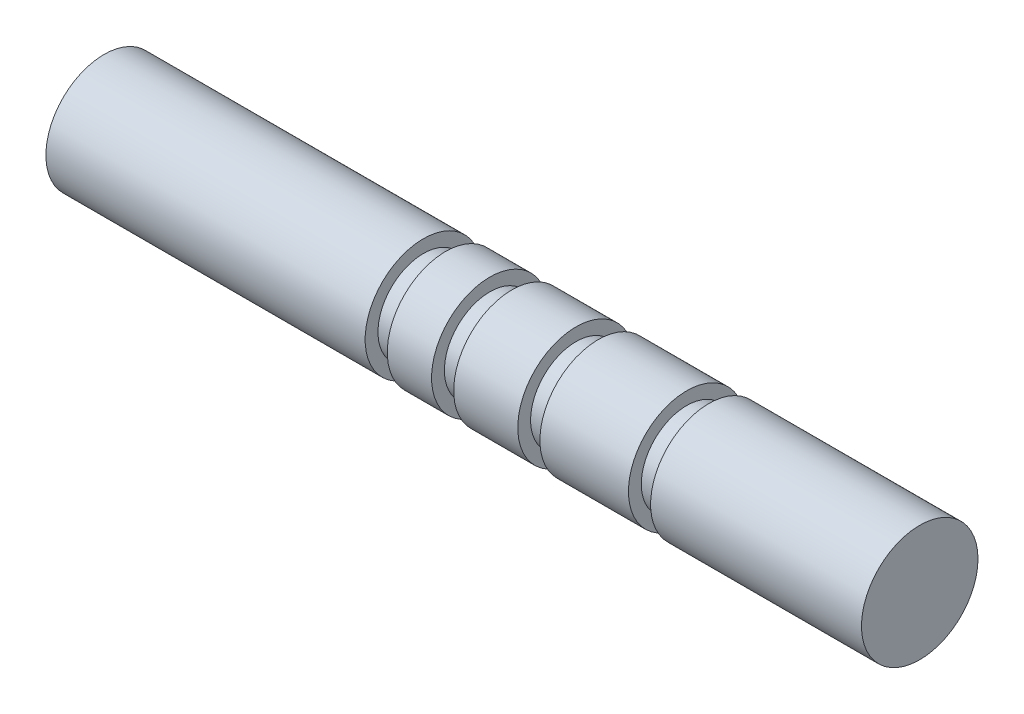
from build123d import *


with BuildPart() as part:
    # Rod Half-Profile Sketch → Grooved Rod Revolve (revolve)
    with BuildSketch(Plane.XY, mode=Mode.PRIVATE) as grooved_rod_revolve_sk:
        Polygon((-44.45, 0), (-44.45, 6.35), (-9.652, 6.35), (-9.652, 4.953), (-7.239, 4.953), (-7.239, 6.35), (-2.413, 6.35), (-2.413, 4.953), (0, 4.953), (0, 6.35), (6.985, 6.35), (6.985, 4.953), (9.398, 4.953), (9.398, 6.35), (19.05, 6.35), (19.05, 4.953), (21.463, 4.953), (21.463, 6.35), (44.45, 6.35), (44.45, 0), align=None)
    revolve(grooved_rod_revolve_sk.sketch.rotate(Axis((49.991353887, 0, 0), (-1, 0, 0)), 90), axis=Axis((49.991353887, 0, 0), (-1, 0, 0)))


solid = part.part
